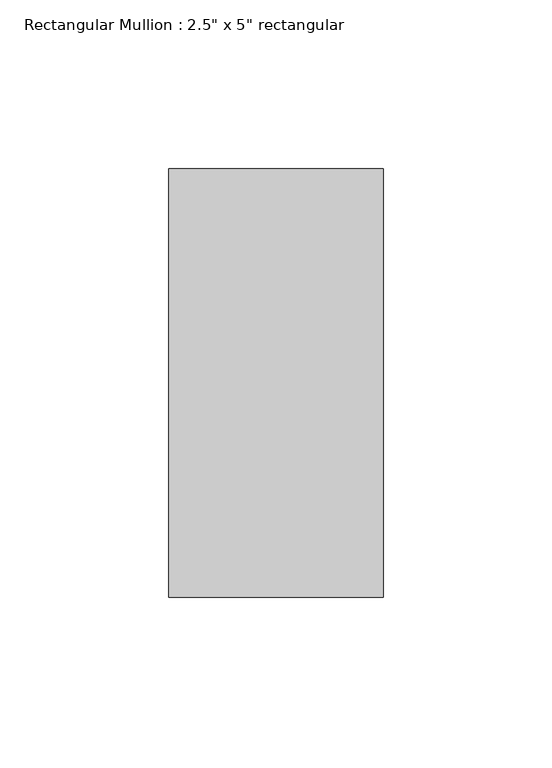
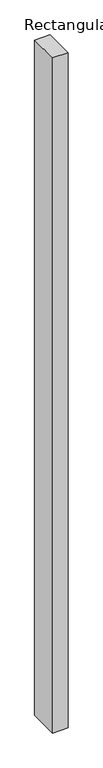
"""IFC4 building model written with IfcOpenShell, lengths in millimetres: member geometry."""

from ifc_helpers import new_model, si_unit, frame, origin, place, context, project, spatial, polyline, outline, extrude, source, transform, mapped, element, save


def member_2ed7bf35(model_context):
    return source(origin(), model_context, "Body", "SweptSolid", [
        extrude(outline(polyline([(31.75, 63.5), (31.75, -63.5), (-31.75, -63.5), (-31.75, 63.5), (31.75, 63.5)])), frame((0.0, 0.0, -2921.0), z_axis=(0.0, 0.0, 1.0), x_axis=(1.0, 0.0, 0.0)), (0.0, 0.0, 1.0), 2921.0),
    ])


if __name__ == "__main__":
    model = new_model("IFC4")
    model_context = context("Model", 3, world=origin())
    ifc_project = project(units=[si_unit("LENGTHUNIT", "METRE", prefix="MILLI")], contexts=[model_context])
    site = spatial("IfcSite", under=ifc_project)
    building = spatial("IfcBuilding", under=site)
    placement = place(None, origin())
    member_shape = member_2ed7bf35(model_context)
    element("IfcMember", 1, ObjectType="Rectangular Mullion : 2.5\" x 5\" rectangular", at=placement, inside=building, context=model_context, shape_type="MappedRepresentation", body=[
        mapped(member_shape, transform((0.0, 0.0, 0.0), x_axis=(1.0, 0.0, 0.0), y_axis=(0.0, 1.0, 0.0), z_axis=(0.0, 0.0, 1.0))),
    ])
    save(model, "model.ifc")

# Revit data of these elements
# Type "Rectangular Mullion : 2.5\" x 5\" rectangular"
#   built-in parameter 1007304 = 0.416667 (stored number, unit not read)
#   built-in parameter 1007301 = 0.104167 (stored number, unit not read)
#   built-in parameter 1007300 = 0.104167 (stored number, unit not read)
# Element 1 (IfcMember, "Rectangular Mullion : 2.5\" x 5\" rectangular")
#   Materials on its faces: "Iron, Ductile"
# Materials
#   "Iron, Ductile": class "Metal", colour RGB 0 0 0, transparency 0, Description = "Ductile cast iron", Cost = 0
